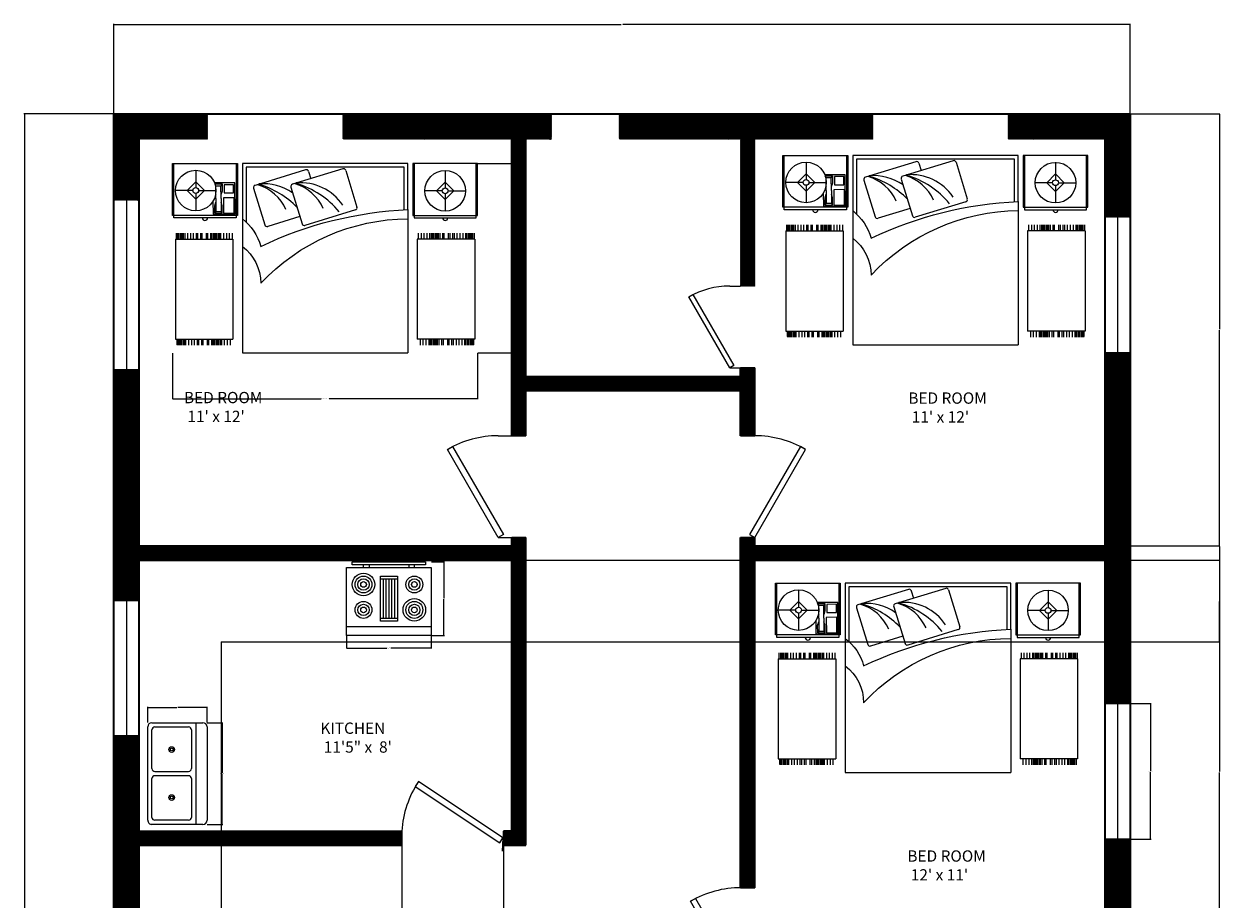
# Model space of a CAD drawing. Units: inches. Extents: x -19 to 404, y -21 to 673.
# Tile 3 of 3: x -19 to 404, y 363 to 673. Entities that reach past the tile are written whole.
import ezdxf

# ---------------------------------------------------------------- set-up
doc = ezdxf.new("R2010")
doc.units = ezdxf.units.IN
doc.header["$MEASUREMENT"] = 0
for name, color, linetype, lineweight in [('A-ANNO-DIMS', 2, 'Continuous', 18), ('A-AREA-IDEN', 7, 'Continuous', 18), ('A-WALL', 7, 'Continuous', 35), ('bedroom', 120, 'Continuous', 18), ('doors', 40, 'Continuous', 18), ('kitchen', 181, 'Continuous', 18), ('window', 30, 'Continuous', 18)]:
    doc.layers.add(name, color=color, linetype=linetype, lineweight=lineweight)
doc.layers.add('A-WALL-PATT', color=244, linetype='Continuous', lineweight=13, true_color=0x991b1e)
doc.styles.get("Standard").update_dxf_attribs({"font": 'arial.ttf'})
doc.dimstyles.get("Standard").update_dxf_attribs({"dimtxt": 0.18, "dimasz": 0.18, "dimexe": 0.18, "dimexo": 0.0625, "dimgap": 0.09, "dimtad": 0, "dimtih": 1, "dimtoh": 1, "dimdec": 4, "dimzin": 0, "dimdsep": 46, "dimtxsty": 'Standard', "dimcen": 0.09, "dimadec": 0, "dimazin": 0, "dimtfac": 1, "dimtdec": 4, "dimtofl": 0, "dimtmove": 0, "dimatfit": 3, "dimfxl": 1, "dimtolj": 1, "dimtzin": 0, "dimarcsym": 0})
pattern_1 = [(45, (-13642.13922, -42713.83606), (-0.08838834765, 0.08838834765), [])]

# ---------------------------------------------------------------- blocks, each defined once
blk = doc.blocks.new('*U5')
for p, q in [((0, 0), (0, -100)), ((750, 0), (750, -100))]:
    blk.add_line(p, q)
blk.add_lwpolyline([(0, 0), (649.5, 375), (671.4, 337.1), (21.9, -37.9)], close=True)
blk.add_arc((0, 0), 750, 0, 30)
blk = doc.blocks.new('*U6')
for p, q in [((0, 0), (0, 100)), ((750, 0), (750, 100))]:
    blk.add_line(p, q)
blk.add_lwpolyline([(0, 0), (649.5, -375), (671.4, -337.1), (21.9, 37.9)], close=True)
blk.add_arc((0, 0), 750, 330, 0)
blk = doc.blocks.new('3')
for p, q in [((185.866, 224.677), (185.866, 225.236)), ((185.866, 225.236), (186.566, 225.236)), ((185.88, 224.649), (185.88, 225.236)), ((186.552, 225.236), (186.552, 224.649)), ((186.566, 225.236), (186.566, 224.677)), ((186.62, 225.236), (186.62, 224.64)), ((188.409, 225.236), (186.62, 225.236)), ((188.409, 224.739), (188.409, 225.236)), ((188.463, 225.236), (188.463, 224.677)), ((189.162, 225.236), (188.463, 225.236)), ((188.477, 225.236), (188.477, 224.649)), ((189.148, 224.649), (189.148, 225.236)), ((189.162, 224.677), (189.162, 225.236)), ((186.116, 225.164), (186.116, 224.976)), ((187.303, 225.168), (186.758, 225.001)), ((187.706, 225.179), (187.161, 225.012)), ((187.334, 225.152), (187.359, 225.073)), ((187.737, 225.163), (187.858, 224.766)), ((188.812, 225.162), (188.812, 224.974)), ((186.084, 224.945), (185.896, 224.945)), ((186.022, 224.945), (186.116, 225.039)), ((186.116, 224.851), (186.022, 224.945)), ((186.116, 225.039), (186.21, 224.945)), ((186.21, 224.945), (186.116, 224.851)), ((186.147, 224.945), (186.335, 224.945)), ((186.54, 225.027), (186.319, 225.027)), ((186.321, 225.017), (186.401, 225.017)), ((186.333, 224.997), (186.321, 225.017)), ((186.334, 224.858), (186.333, 224.997)), ((186.333, 224.997), (186.389, 224.997)), ((186.401, 225.017), (186.389, 224.997)), ((186.39, 224.858), (186.389, 224.997)), ((186.401, 224.938), (186.389, 224.898)), ((186.401, 225.017), (186.401, 224.938)), ((186.541, 224.69), (186.54, 225.027)), ((186.742, 224.97), (186.863, 224.573)), ((187.144, 224.981), (187.266, 224.584)), ((188.781, 224.942), (188.593, 224.942)), ((188.812, 225.036), (188.718, 224.942)), ((188.718, 224.942), (188.812, 224.848)), ((188.907, 224.942), (188.812, 225.036)), ((188.812, 224.848), (188.907, 224.942)), ((188.844, 224.942), (189.032, 224.942)), ((186.116, 224.914), (186.116, 224.726)), ((186.302, 224.83), (186.303, 224.689)), ((186.322, 224.779), (186.334, 224.818)), ((186.331, 224.905), (186.334, 224.898)), ((186.334, 224.858), (186.334, 224.719)), ((186.39, 224.858), (186.39, 224.719)), ((186.402, 224.779), (186.39, 224.819)), ((188.812, 224.911), (188.812, 224.723)), ((186.566, 224.677), (185.866, 224.677)), ((186.303, 224.689), (186.541, 224.69)), ((186.323, 224.699), (186.322, 224.779)), ((186.334, 224.719), (186.323, 224.699)), ((186.323, 224.699), (186.402, 224.7)), ((186.334, 224.719), (186.39, 224.719)), ((186.402, 224.7), (186.39, 224.719)), ((186.402, 224.7), (186.402, 224.779)), ((187.842, 224.735), (187.297, 224.568)), ((188.409, 224.739), (188.409, 223.191)), ((188.463, 224.677), (189.162, 224.677)), ((186.552, 224.649), (185.88, 224.649)), ((186.62, 224.64), (186.62, 223.191)), ((187.242, 224.663), (186.894, 224.557)), ((188.477, 224.649), (189.148, 224.649)), ((185.897, 224.42, -0.909), (185.897, 223.338, -0.909)), ((185.897, 224.42, -0.909), (186.517, 224.42, -0.909)), ((185.904, 224.485, -0.909), (185.904, 224.42, -0.909)), ((185.92, 224.485, -0.909), (185.92, 224.42, -0.909)), ((185.92, 224.485, -0.909), (185.92, 224.42, -0.909)), ((185.935, 224.485, -0.909), (185.935, 224.42, -0.909)), ((185.951, 224.485, -0.909), (185.951, 224.42, -0.909)), ((185.966, 224.485, -0.909), (185.966, 224.42, -0.909)), ((185.982, 224.485, -0.909), (185.982, 224.42, -0.909)), ((185.997, 224.485, -0.909), (185.997, 224.42, -0.909)), ((186.028, 224.485, -0.909), (186.028, 224.42, -0.909)), ((186.059, 224.485, -0.909), (186.059, 224.42, -0.909)), ((186.09, 224.485, -0.909), (186.09, 224.42, -0.909)), ((186.09, 224.485, -0.909), (186.09, 224.42, -0.909)), ((186.121, 224.485, -0.909), (186.121, 224.42, -0.909)), ((186.137, 224.485, -0.909), (186.137, 224.42, -0.909)), ((186.168, 224.485, -0.909), (186.168, 224.42, -0.909)), ((186.183, 224.485, -0.909), (186.183, 224.42, -0.909)), ((186.23, 224.485, -0.909), (186.23, 224.42, -0.909)), ((186.245, 224.485, -0.909), (186.245, 224.42, -0.909)), ((186.276, 224.485, -0.909), (186.276, 224.42, -0.909)), ((186.292, 224.485, -0.909), (186.292, 224.42, -0.909)), ((186.307, 224.485, -0.909), (186.307, 224.42, -0.909)), ((186.323, 224.485, -0.909), (186.323, 224.42, -0.909)), ((186.338, 224.485, -0.909), (186.338, 224.42, -0.909)), ((186.354, 224.485, -0.909), (186.354, 224.42, -0.909)), ((186.369, 224.485, -0.909), (186.369, 224.42, -0.909)), ((186.385, 224.485, -0.909), (186.385, 224.42, -0.909)), ((186.416, 224.485, -0.909), (186.416, 224.42, -0.909)), ((186.447, 224.485, -0.909), (186.447, 224.42, -0.909)), ((186.478, 224.485, -0.909), (186.478, 224.42, -0.909)), ((186.509, 224.485, -0.909), (186.509, 224.42, -0.909)), ((186.517, 224.42, -0.909), (186.517, 223.338, -0.909)), ((189.131, 224.42, -0.909), (188.511, 224.42, -0.909)), ((188.511, 224.42, -0.909), (188.511, 223.338, -0.909)), ((188.52, 224.485, -0.909), (188.52, 224.42, -0.909)), ((188.551, 224.485, -0.909), (188.551, 224.42, -0.909)), ((188.582, 224.485, -0.909), (188.582, 224.42, -0.909)), ((188.613, 224.485, -0.909), (188.613, 224.42, -0.909)), ((188.644, 224.485, -0.909), (188.644, 224.42, -0.909)), ((188.66, 224.485, -0.909), (188.66, 224.42, -0.909)), ((188.675, 224.485, -0.909), (188.675, 224.42, -0.909)), ((188.691, 224.485, -0.909), (188.691, 224.42, -0.909)), ((188.706, 224.485, -0.909), (188.706, 224.42, -0.909)), ((188.722, 224.485, -0.909), (188.722, 224.42, -0.909)), ((188.737, 224.485, -0.909), (188.737, 224.42, -0.909)), ((188.753, 224.485, -0.909), (188.753, 224.42, -0.909)), ((188.784, 224.485, -0.909), (188.784, 224.42, -0.909)), ((188.799, 224.485, -0.909), (188.799, 224.42, -0.909)), ((188.846, 224.485, -0.909), (188.846, 224.42, -0.909)), ((188.861, 224.485, -0.909), (188.861, 224.42, -0.909)), ((188.892, 224.485, -0.909), (188.892, 224.42, -0.909)), ((188.908, 224.485, -0.909), (188.908, 224.42, -0.909)), ((188.939, 224.485, -0.909), (188.939, 224.42, -0.909)), ((188.939, 224.485, -0.909), (188.939, 224.42, -0.909)), ((188.97, 224.485, -0.909), (188.97, 224.42, -0.909)), ((189.001, 224.485, -0.909), (189.001, 224.42, -0.909)), ((189.032, 224.485, -0.909), (189.032, 224.42, -0.909)), ((189.047, 224.485, -0.909), (189.047, 224.42, -0.909)), ((189.063, 224.485, -0.909), (189.063, 224.42, -0.909)), ((189.078, 224.485, -0.909), (189.078, 224.42, -0.909)), ((189.094, 224.485, -0.909), (189.094, 224.42, -0.909)), ((189.109, 224.485, -0.909), (189.109, 224.42, -0.909)), ((189.109, 224.485, -0.909), (189.109, 224.42, -0.909)), ((189.125, 224.485, -0.909), (189.125, 224.42, -0.909)), ((189.131, 224.42, -0.909), (189.131, 223.338, -0.909)), ((185.897, 223.338, -0.909), (186.517, 223.338, -0.909)), ((185.911, 223.338, -0.909), (185.911, 223.279, -0.909)), ((185.911, 223.338, -0.909), (185.911, 223.279, -0.909)), ((185.911, 223.338, -0.909), (185.911, 223.279, -0.909)), ((185.914, 223.338, -0.909), (185.914, 223.273, -0.909)), ((185.929, 223.338, -0.909), (185.929, 223.273, -0.909)), ((185.929, 223.338, -0.909), (185.929, 223.273, -0.909)), ((185.945, 223.338, -0.909), (185.945, 223.273, -0.909)), ((185.96, 223.338, -0.909), (185.96, 223.273, -0.909)), ((185.976, 223.338, -0.909), (185.976, 223.273, -0.909)), ((185.991, 223.338, -0.909), (185.991, 223.273, -0.909)), ((186.007, 223.338, -0.909), (186.007, 223.273, -0.909)), ((186.038, 223.338, -0.909), (186.038, 223.273, -0.909)), ((186.069, 223.338, -0.909), (186.069, 223.273, -0.909)), ((186.1, 223.338, -0.909), (186.1, 223.273, -0.909)), ((186.1, 223.338, -0.909), (186.1, 223.273, -0.909)), ((186.131, 223.338, -0.909), (186.131, 223.273, -0.909)), ((186.146, 223.338, -0.909), (186.146, 223.273, -0.909)), ((186.177, 223.338, -0.909), (186.177, 223.273, -0.909)), ((186.193, 223.338, -0.909), (186.193, 223.273, -0.909)), ((186.239, 223.338, -0.909), (186.239, 223.273, -0.909)), ((186.255, 223.338, -0.909), (186.255, 223.273, -0.909)), ((186.286, 223.338, -0.909), (186.286, 223.273, -0.909)), ((186.301, 223.338, -0.909), (186.301, 223.273, -0.909)), ((186.317, 223.338, -0.909), (186.317, 223.273, -0.909)), ((186.332, 223.338, -0.909), (186.332, 223.273, -0.909)), ((186.348, 223.338, -0.909), (186.348, 223.273, -0.909)), ((186.363, 223.338, -0.909), (186.363, 223.273, -0.909)), ((186.379, 223.338, -0.909), (186.379, 223.273, -0.909)), ((186.394, 223.338, -0.909), (186.394, 223.273, -0.909)), ((186.425, 223.338, -0.909), (186.425, 223.273, -0.909)), ((186.456, 223.338, -0.909), (186.456, 223.273, -0.909)), ((186.487, 223.338, -0.909), (186.487, 223.273, -0.909)), ((189.131, 223.338, -0.909), (188.511, 223.338, -0.909)), ((188.541, 223.338, -0.909), (188.541, 223.273, -0.909)), ((188.572, 223.338, -0.909), (188.572, 223.273, -0.909)), ((188.603, 223.338, -0.909), (188.603, 223.273, -0.909)), ((188.634, 223.338, -0.909), (188.634, 223.273, -0.909)), ((188.65, 223.338, -0.909), (188.65, 223.273, -0.909)), ((188.665, 223.338, -0.909), (188.665, 223.273, -0.909)), ((188.681, 223.338, -0.909), (188.681, 223.273, -0.909)), ((188.696, 223.338, -0.909), (188.696, 223.273, -0.909)), ((188.712, 223.338, -0.909), (188.712, 223.273, -0.909)), ((188.727, 223.338, -0.909), (188.727, 223.273, -0.909)), ((188.743, 223.338, -0.909), (188.743, 223.273, -0.909)), ((188.774, 223.338, -0.909), (188.774, 223.273, -0.909)), ((188.789, 223.338, -0.909), (188.789, 223.273, -0.909)), ((188.836, 223.338, -0.909), (188.836, 223.273, -0.909)), ((188.851, 223.338, -0.909), (188.851, 223.273, -0.909)), ((188.882, 223.338, -0.909), (188.882, 223.273, -0.909)), ((188.898, 223.338, -0.909), (188.898, 223.273, -0.909)), ((188.929, 223.338, -0.909), (188.929, 223.273, -0.909)), ((188.929, 223.338, -0.909), (188.929, 223.273, -0.909)), ((188.96, 223.338, -0.909), (188.96, 223.273, -0.909)), ((188.991, 223.338, -0.909), (188.991, 223.273, -0.909)), ((189.022, 223.338, -0.909), (189.022, 223.273, -0.909)), ((189.037, 223.338, -0.909), (189.037, 223.273, -0.909)), ((189.053, 223.338, -0.909), (189.053, 223.273, -0.909)), ((189.068, 223.338, -0.909), (189.068, 223.273, -0.909)), ((189.084, 223.338, -0.909), (189.084, 223.273, -0.909)), ((189.099, 223.338, -0.909), (189.099, 223.273, -0.909)), ((189.099, 223.338, -0.909), (189.099, 223.273, -0.909)), ((189.115, 223.338, -0.909), (189.115, 223.273, -0.909)), ((189.117, 223.338, -0.909), (189.117, 223.279, -0.909)), ((189.117, 223.338, -0.909), (189.117, 223.279, -0.909)), ((189.117, 223.338, -0.909), (189.117, 223.279, -0.909)), ((186.62, 223.191), (188.409, 223.191))]:
    blk.add_line(p, q)
blk.add_lwpolyline([(188.369, 224.737), (188.369, 225.197), (186.66, 225.197), (186.66, 224.606)])
for points in [[(186.422, 225.007), (186.422, 224.92), (186.525, 224.92), (186.525, 225.008)], [(186.415, 224.866), (186.416, 224.7), (186.531, 224.7), (186.53, 224.867)]]:
    blk.add_lwpolyline(points, close=True)
for points in [[(186.62, 224.64, -0.162278), (186.819, 224.342, -0.100664), (188.409, 224.739, -0.100664)], [(186.62, 224.342, -0.236068), (186.819, 223.944, -0.205258), (188.409, 224.64, -0.205258)]]:
    blk.add_lwpolyline(points, format="xyb")
for centre, radius in [((186.116, 224.945), 0.219), ((188.812, 224.942), 0.219), ((186.116, 224.945), 0.0313), ((188.812, 224.942), 0.0313)]:
    blk.add_circle(centre, radius)
for centre, radius, start, end in [((187.311, 225.145), 0.0248, 17.0142, 107.0142), ((187.713, 225.156), 0.0248, 17.0142, 107.0142), ((186.765, 224.978), 0.0248, 107.0142, 197.0142), ((186.647, 224.541), 0.487, 24.2209, 73.0691), ((186.848, 224.471), 0.547, 54.6851, 95.1605), ((186.536, 224.105), 0.943, 44.2727, 73.7189), ((187.168, 224.989), 0.0248, 107.0142, 197.0142), ((187.05, 224.552), 0.487, 24.2209, 73.0691), ((187.25, 224.482), 0.547, 33.7801, 95.1605), ((186.938, 224.116), 0.943, 39.4023, 73.7189), ((187.835, 224.758), 0.0248, 287.0142, 17.0142), ((186.216, 224.649), 0.028, 180, 0), ((186.887, 224.581), 0.0248, 197.0142, 287.0142), ((187.289, 224.592), 0.0248, 197.0142, 287.0142), ((188.812, 224.649), 0.028, 180, 0)]:
    blk.add_arc(centre, radius, start, end)
blk = doc.blocks.new('Sink-double - 36 in top')
for p, q in [((-18, -4), (18, -4)), ((-0.75, -18.5), (-0.75, -6.5)), ((0.75, -6.5), (0.75, -18.5))]:
    blk.add_line(p, q)
for points in [[(-16.5, 0), (16.5, 0)], [(-18, -19.5), (-18, -1.5)], [(18, -1.5), (18, -19.5)], [(-16.5, -18.5), (-16.5, -6.5)], [(-15.5, -5.5), (-1.75, -5.5)], [(1.75, -5.5), (15.5, -5.5)], [(16.5, -6.5), (16.5, -18.5)], [(16.5, -21), (-16.5, -21)], [(-1.75, -19.5), (-15.5, -19.5)], [(15.5, -19.5), (1.75, -19.5)]]:
    blk.add_lwpolyline(points)
for centre, radius in [((-8.5, -12.5), 1), ((-8.5, -12.5), 0.5), ((8.5, -12.5), 1), ((8.5, -12.5), 0.5)]:
    blk.add_circle(centre, radius)
for centre, radius, start, end in [((-16.5, -1.5), 1.5, 90, 180), ((16.5, -1.5), 1.5, 0, 90), ((-15.5, -6.5), 1, 90, 180), ((-1.75, -6.5), 1, 0, 90), ((1.75, -6.5), 1, 90, 180), ((15.5, -6.5), 1, 0, 90), ((-16.5, -19.5), 1.5, 180, 270), ((-15.5, -18.5), 1, 180, 270), ((-1.75, -18.5), 1, 270, 0), ((1.75, -18.5), 1, 180, 270), ((15.5, -18.5), 1, 270, 0), ((16.5, -19.5), 1.5, 270, 0)]:
    blk.add_arc(centre, radius, start, end)
blk = doc.blocks.new('Range-Oven - 30 in top')
for p, q in [((0, -3), (30, -3)), ((12, -6), (18, -6)), ((13, -20), (13, -6)), ((14, -6), (14, -20)), ((15, -20), (15, -6)), ((16, -6), (16, -20)), ((17, -20), (17, -6)), ((18, -20), (12, -20)), ((6, -24), (6, -25)), ((8, -25), (8, -24)), ((22, -25), (22, -24)), ((24, -24), (24, -25))]:
    blk.add_line(p, q)
for points in [[(0, -24), (0, 0), (30, 0), (30, -24)], [(12, -21), (12, -5), (18, -5), (18, -21)], [(2, -26), (2, -25), (28, -25), (28, -26)]]:
    blk.add_lwpolyline(points, close=True)
for centre, radius in [((6, -9), 4), ((6, -9), 3), ((6, -9), 2), ((6, -9), 1), ((24, -9), 3), ((24, -9), 2), ((24, -9), 1), ((6, -18), 3), ((6, -18), 2), ((24, -18), 4), ((24, -18), 3), ((24, -18), 2), ((6, -18), 1), ((24, -18), 1)]:
    blk.add_circle(centre, radius)
blk = doc.blocks.new('WIN-48IN')
for p, q in [((0, 48), (9, 48)), ((0, 0), (0, 48)), ((0, 48), (4.5, 48)), ((4.5, 48), (4.5, 0)), ((9, 48), (9, 0)), ((9, 0), (0, 0))]:
    blk.add_line(p, q)
blk = doc.blocks.new('*D11')
at = {"layer": 'A-ANNO-DIMS', "color": 0, "lineweight": -2, "transparency": 16777216}
for p, q in [((33.51, 556.07), (33.51, 539.75)), ((141.51, 556.07), (141.51, 539.75)), ((33.69, 539.93), (86.12, 539.93)), ((141.33, 539.93), (88.89, 539.93))]:
    blk.add_line(p, q, dxfattribs=at)
at = {"layer": 'A-ANNO-DIMS', "color": 0, "transparency": 16777216}
for points in [[(33.69, 539.96), (33.69, 539.9), (33.51, 539.93)], [(141.33, 539.96), (141.33, 539.9), (141.51, 539.93)]]:
    blk.add_solid(points, dxfattribs=at)
at = {"layer": 'Defpoints', "color": 0, "transparency": 16777216}
for p in [(33.51, 556.13), (141.51, 556.13), (141.51, 539.93)]:
    blk.add_point(p, dxfattribs=at)
at = {"layer": 'A-ANNO-DIMS', "color": 0, "transparency": 16777216, "insert": (87.51, 539.93), "char_height": 0.18, "attachment_point": 5}
blk.add_mtext('\\A1;BED GROUP 108 TYP.', dxfattribs=at)
blk = doc.blocks.new('*D12')
at = {"layer": 'A-ANNO-DIMS', "color": 0, "lineweight": -2, "transparency": 16777216}
for p, q in [((141.57, 623.16), (157.89, 623.16)), ((157.71, 622.98), (157.71, 589.83)), ((157.71, 556.31), (157.71, 589.46)), ((141.57, 556.13), (157.89, 556.13))]:
    blk.add_line(p, q, dxfattribs=at)
at = {"layer": 'A-ANNO-DIMS', "color": 0, "transparency": 16777216}
for points in [[(157.68, 622.98), (157.74, 622.98), (157.71, 623.16)], [(157.68, 556.31), (157.74, 556.31), (157.71, 556.13)]]:
    blk.add_solid(points, dxfattribs=at)
at = {"layer": 'Defpoints', "color": 0, "transparency": 16777216}
for p in [(141.51, 623.16), (157.71, 623.16), (141.51, 556.13)]:
    blk.add_point(p, dxfattribs=at)
at = {"layer": 'A-ANNO-DIMS', "color": 0, "transparency": 16777216, "insert": (157.71, 589.64), "char_height": 0.18, "attachment_point": 5}
blk.add_mtext('\\A1;67 TYP.', dxfattribs=at)
blk = doc.blocks.new('*D13')
at = {"layer": 'A-ANNO-DIMS', "color": 0, "lineweight": -2, "transparency": 16777216}
for p, q in [((372.71, 431.98), (380.03, 431.98)), ((379.85, 431.8), (379.85, 408.17)), ((379.85, 384.16), (379.85, 407.8)), ((372.71, 383.98), (380.03, 383.98))]:
    blk.add_line(p, q, dxfattribs=at)
at = {"layer": 'A-ANNO-DIMS', "color": 0, "transparency": 16777216}
for points in [[(379.82, 431.8), (379.88, 431.8), (379.85, 431.98)], [(379.82, 384.16), (379.88, 384.16), (379.85, 383.98)]]:
    blk.add_solid(points, dxfattribs=at)
at = {"layer": 'Defpoints', "color": 0, "transparency": 16777216}
for p in [(372.65, 431.98), (379.85, 431.98), (372.65, 383.98)]:
    blk.add_point(p, dxfattribs=at)
at = {"layer": 'A-ANNO-DIMS', "color": 0, "transparency": 16777216, "insert": (379.85, 407.98), "char_height": 0.18, "attachment_point": 5}
blk.add_mtext('\\A1;WINDOW 48 TYP.', dxfattribs=at)
blk = doc.blocks.new('*D14')
at = {"layer": 'A-ANNO-DIMS', "color": 0, "lineweight": -2, "transparency": 16777216}
for p, q in [((363.65, 383.92), (363.65, 376.6)), ((372.65, 383.92), (372.65, 376.6)), ((363.83, 376.78), (367.69, 376.78)), ((372.47, 376.78), (368.61, 376.78))]:
    blk.add_line(p, q, dxfattribs=at)
at = {"layer": 'A-ANNO-DIMS', "color": 0, "transparency": 16777216}
for points in [[(363.83, 376.81), (363.83, 376.75), (363.65, 376.78)], [(372.47, 376.81), (372.47, 376.75), (372.65, 376.78)]]:
    blk.add_solid(points, dxfattribs=at)
at = {"layer": 'Defpoints', "color": 0, "transparency": 16777216}
for p in [(363.65, 383.98), (372.65, 383.98), (372.65, 376.78)]:
    blk.add_point(p, dxfattribs=at)
at = {"layer": 'A-ANNO-DIMS', "color": 0, "transparency": 16777216, "insert": (368.15, 376.78), "char_height": 0.18, "attachment_point": 5}
blk.add_mtext('\\A1;9 TYP.', dxfattribs=at)
blk = doc.blocks.new('*D21')
at = {"layer": 'A-ANNO-DIMS', "color": 0, "lineweight": -2, "transparency": 16777216}
for p, q in [((45.75, 425.23), (51.27, 425.23)), ((51.09, 425.05), (51.09, 407.41)), ((51.09, 389.41), (51.09, 407.04)), ((45.75, 389.23), (51.27, 389.23))]:
    blk.add_line(p, q, dxfattribs=at)
at = {"layer": 'A-ANNO-DIMS', "color": 0, "transparency": 16777216}
for points in [[(51.06, 425.05), (51.12, 425.05), (51.09, 425.23)], [(51.06, 389.41), (51.12, 389.41), (51.09, 389.23)]]:
    blk.add_solid(points, dxfattribs=at)
at = {"layer": 'Defpoints', "color": 0, "transparency": 16777216}
for p in [(45.69, 425.23), (45.69, 389.23), (51.09, 389.23)]:
    blk.add_point(p, dxfattribs=at)
at = {"layer": 'A-ANNO-DIMS', "color": 0, "transparency": 16777216, "insert": (51.09, 407.23), "char_height": 0.18, "attachment_point": 5}
blk.add_mtext('\\A1;DOUBLE SINK 36', dxfattribs=at)
blk = doc.blocks.new('*D22')
at = {"layer": 'A-ANNO-DIMS', "color": 0, "lineweight": -2, "transparency": 16777216}
for p, q in [((24.69, 425.29), (24.69, 430.81)), ((24.87, 430.63), (34.99, 430.63)), ((45.51, 430.63), (35.39, 430.63)), ((45.69, 425.29), (45.69, 430.81))]:
    blk.add_line(p, q, dxfattribs=at)
at = {"layer": 'A-ANNO-DIMS', "color": 0, "transparency": 16777216}
for points in [[(24.87, 430.66), (24.87, 430.6), (24.69, 430.63)], [(45.51, 430.66), (45.51, 430.6), (45.69, 430.63)]]:
    blk.add_solid(points, dxfattribs=at)
at = {"layer": 'Defpoints', "color": 0, "transparency": 16777216}
for p in [(45.69, 430.63), (24.69, 425.23), (45.69, 425.23)]:
    blk.add_point(p, dxfattribs=at)
at = {"layer": 'A-ANNO-DIMS', "color": 0, "transparency": 16777216, "insert": (35.19, 430.63), "char_height": 0.18, "attachment_point": 5}
blk.add_mtext('\\A1;21', dxfattribs=at)
blk = doc.blocks.new('*D23')
at = {"layer": 'A-ANNO-DIMS', "color": 0, "lineweight": -2, "transparency": 16777216}
for p, q in [((95.11, 456.1), (95.11, 451.48)), ((125.11, 456.1), (125.11, 451.48)), ((95.29, 451.66), (109.42, 451.66)), ((124.93, 451.66), (110.81, 451.66))]:
    blk.add_line(p, q, dxfattribs=at)
at = {"layer": 'A-ANNO-DIMS', "color": 0, "transparency": 16777216}
for points in [[(95.29, 451.69), (95.29, 451.63), (95.11, 451.66)], [(124.93, 451.69), (124.93, 451.63), (125.11, 451.66)]]:
    blk.add_solid(points, dxfattribs=at)
at = {"layer": 'Defpoints', "color": 0, "transparency": 16777216}
for p in [(95.11, 456.16), (125.11, 456.16), (95.11, 451.66)]:
    blk.add_point(p, dxfattribs=at)
at = {"layer": 'A-ANNO-DIMS', "color": 0, "transparency": 16777216, "insert": (110.11, 451.66), "char_height": 0.18, "attachment_point": 5}
blk.add_mtext('\\A1;RANGE 30', dxfattribs=at)
blk = doc.blocks.new('*D24')
at = {"layer": 'A-ANNO-DIMS', "color": 0, "lineweight": -2, "transparency": 16777216}
for p, q in [((125.17, 482.16), (129.79, 482.16)), ((129.61, 481.98), (129.61, 469.35)), ((129.61, 456.34), (129.61, 468.98)), ((125.17, 456.16), (129.79, 456.16))]:
    blk.add_line(p, q, dxfattribs=at)
at = {"layer": 'A-ANNO-DIMS', "color": 0, "transparency": 16777216}
for points in [[(129.58, 481.98), (129.64, 481.98), (129.61, 482.16)], [(129.58, 456.34), (129.64, 456.34), (129.61, 456.16)]]:
    blk.add_solid(points, dxfattribs=at)
at = {"layer": 'Defpoints', "color": 0, "transparency": 16777216}
for p in [(125.11, 482.16), (125.11, 456.16), (129.61, 456.16)]:
    blk.add_point(p, dxfattribs=at)
at = {"layer": 'A-ANNO-DIMS', "color": 0, "transparency": 16777216, "insert": (129.61, 469.16), "char_height": 0.18, "attachment_point": 5}
blk.add_mtext('\\A1;26', dxfattribs=at)
blk = doc.blocks.new('*D25')
at = {"layer": 'A-ANNO-DIMS', "color": 0, "lineweight": -2, "transparency": 16777216}
for p, q in [((12.65, 640.88), (12.65, 672.6)), ((12.83, 672.42), (192.36, 672.42)), ((372.47, 672.42), (192.94, 672.42)), ((372.65, 640.88), (372.65, 672.6))]:
    blk.add_line(p, q, dxfattribs=at)
at = {"layer": 'A-ANNO-DIMS', "color": 0, "transparency": 16777216}
for points in [[(12.83, 672.45), (12.83, 672.39), (12.65, 672.42)], [(372.47, 672.45), (372.47, 672.39), (372.65, 672.42)]]:
    blk.add_solid(points, dxfattribs=at)
at = {"layer": 'Defpoints', "color": 0, "transparency": 16777216}
for p in [(372.65, 672.42), (12.65, 640.82), (372.65, 640.82)]:
    blk.add_point(p, dxfattribs=at)
at = {"layer": 'A-ANNO-DIMS', "color": 0, "transparency": 16777216, "insert": (192.65, 672.42), "char_height": 0.18, "attachment_point": 5}
blk.add_mtext('\\A1;360', dxfattribs=at)
blk = doc.blocks.new('*D26')
at = {"layer": 'A-ANNO-DIMS', "color": 0, "lineweight": -2, "transparency": 16777216}
for p, q in [((12.59, 640.82), (-19.13, 640.82)), ((-18.95, 640.64), (-18.95, 326)), ((-18.95, 11), (-18.95, 325.64)), ((114.59, 10.82), (-19.13, 10.82))]:
    blk.add_line(p, q, dxfattribs=at)
at = {"layer": 'A-ANNO-DIMS', "color": 0, "transparency": 16777216}
for points in [[(-18.98, 640.64), (-18.92, 640.64), (-18.95, 640.82)], [(-18.98, 11), (-18.92, 11), (-18.95, 10.82)]]:
    blk.add_solid(points, dxfattribs=at)
at = {"layer": 'Defpoints', "color": 0, "transparency": 16777216}
for p in [(12.65, 640.82), (-18.95, 10.82), (114.65, 10.82)]:
    blk.add_point(p, dxfattribs=at)
at = {"layer": 'A-ANNO-DIMS', "color": 0, "transparency": 16777216, "insert": (-18.95, 325.82), "char_height": 0.18, "attachment_point": 5}
blk.add_mtext('\\A1;630', dxfattribs=at)
blk = doc.blocks.new('*D32')
at = {"layer": 'A-ANNO-DIMS', "color": 0, "lineweight": -2, "transparency": 16777216}
for p, q in [((372.71, 640.82), (404.42, 640.82)), ((404.24, 640.64), (404.24, 564.5)), ((404.24, 488), (404.24, 564.14)), ((363.71, 487.82), (404.42, 487.82))]:
    blk.add_line(p, q, dxfattribs=at)
at = {"layer": 'A-ANNO-DIMS', "color": 0, "transparency": 16777216}
for points in [[(404.21, 640.64), (404.27, 640.64), (404.24, 640.82)], [(404.21, 488), (404.27, 488), (404.24, 487.82)]]:
    blk.add_solid(points, dxfattribs=at)
at = {"layer": 'Defpoints', "color": 0, "transparency": 16777216}
for p in [(372.65, 640.82), (404.24, 640.82), (363.65, 487.82)]:
    blk.add_point(p, dxfattribs=at)
at = {"layer": 'A-ANNO-DIMS', "color": 0, "transparency": 16777216, "insert": (404.24, 564.32), "char_height": 0.18, "attachment_point": 5}
blk.add_mtext('\\A1;153', dxfattribs=at)
blk = doc.blocks.new('*D33')
at = {"layer": 'A-ANNO-DIMS', "color": 0, "lineweight": -2, "transparency": 16777216}
for p, q in [((363.71, 487.82), (404.42, 487.82)), ((404.24, 487.64), (404.24, 408)), ((404.24, 328), (404.24, 407.64)), ((363.71, 327.82), (404.42, 327.82))]:
    blk.add_line(p, q, dxfattribs=at)
at = {"layer": 'A-ANNO-DIMS', "color": 0, "transparency": 16777216}
for points in [[(404.21, 487.64), (404.27, 487.64), (404.24, 487.82)], [(404.21, 328), (404.27, 328), (404.24, 327.82)]]:
    blk.add_solid(points, dxfattribs=at)
at = {"layer": 'Defpoints', "color": 0, "transparency": 16777216}
for p in [(363.65, 487.82), (404.24, 487.82), (363.65, 327.82)]:
    blk.add_point(p, dxfattribs=at)
at = {"layer": 'A-ANNO-DIMS', "color": 0, "transparency": 16777216, "insert": (404.24, 407.82), "char_height": 0.18, "attachment_point": 5}
blk.add_mtext('\\A1;160', dxfattribs=at)
blk = doc.blocks.new('*D38')
at = {"layer": 'A-ANNO-DIMS', "color": 0, "lineweight": -2, "transparency": 16777216}
for p, q in [((21.65, 386.76), (21.65, -20.95)), ((50.65, 386.76), (50.65, -20.95)), ((21.83, -20.77), (35.93, -20.77)), ((50.47, -20.77), (36.37, -20.77))]:
    blk.add_line(p, q, dxfattribs=at)
at = {"layer": 'A-ANNO-DIMS', "color": 0, "transparency": 16777216}
for points in [[(21.83, -20.74), (21.83, -20.8), (21.65, -20.77)], [(50.47, -20.74), (50.47, -20.8), (50.65, -20.77)]]:
    blk.add_solid(points, dxfattribs=at)
at = {"layer": 'Defpoints', "color": 0, "transparency": 16777216}
for p in [(21.65, 386.82), (50.65, 386.82), (50.65, -20.77)]:
    blk.add_point(p, dxfattribs=at)
at = {"layer": 'A-ANNO-DIMS', "color": 0, "transparency": 16777216, "insert": (36.15, -20.77), "char_height": 0.18, "attachment_point": 5}
blk.add_mtext('\\A1;29', dxfattribs=at)
blk = doc.blocks.new('*D39')
at = {"layer": 'A-ANNO-DIMS', "color": 0, "lineweight": -2, "transparency": 16777216}
for p, q in [((153.71, 482.82), (404.42, 482.82)), ((404.24, 482.64), (404.24, 468.5)), ((404.24, 454), (404.24, 468.14)), ((153.71, 453.82), (404.42, 453.82))]:
    blk.add_line(p, q, dxfattribs=at)
at = {"layer": 'A-ANNO-DIMS', "color": 0, "transparency": 16777216}
for points in [[(404.21, 482.64), (404.27, 482.64), (404.24, 482.82)], [(404.21, 454), (404.27, 454), (404.24, 453.82)]]:
    blk.add_solid(points, dxfattribs=at)
at = {"layer": 'Defpoints', "color": 0, "transparency": 16777216}
for p in [(153.65, 482.82), (404.24, 482.82), (153.65, 453.82)]:
    blk.add_point(p, dxfattribs=at)
at = {"layer": 'A-ANNO-DIMS', "color": 0, "transparency": 16777216, "insert": (404.24, 468.32), "char_height": 0.18, "attachment_point": 5}
blk.add_mtext('\\A1;29', dxfattribs=at)
blk = doc.blocks.new('*D40')
at = {"layer": 'A-ANNO-DIMS', "color": 0, "lineweight": -2, "transparency": 16777216}
for p, q in [((114.65, 381.76), (114.65, -20.95)), ((150.65, 381.76), (150.65, -20.95)), ((114.83, -20.77), (132.43, -20.77)), ((150.47, -20.77), (132.87, -20.77))]:
    blk.add_line(p, q, dxfattribs=at)
at = {"layer": 'A-ANNO-DIMS', "color": 0, "transparency": 16777216}
for points in [[(114.83, -20.74), (114.83, -20.8), (114.65, -20.77)], [(150.47, -20.74), (150.47, -20.8), (150.65, -20.77)]]:
    blk.add_solid(points, dxfattribs=at)
at = {"layer": 'Defpoints', "color": 0, "transparency": 16777216}
for p in [(114.65, 381.82), (150.65, 381.82), (150.65, -20.77)]:
    blk.add_point(p, dxfattribs=at)
at = {"layer": 'A-ANNO-DIMS', "color": 0, "transparency": 16777216, "insert": (132.65, -20.77), "char_height": 0.18, "attachment_point": 5}
blk.add_mtext('\\A1;36', dxfattribs=at)

msp = doc.modelspace()

# ---------------------------------------------------------------- hatches: boundary and pattern name
at = {"layer": 'A-WALL-PATT'}
h = msp.add_hatch(dxfattribs=at)
h.set_pattern_fill('ANSI31', color=256)
h.set_pattern_definition(pattern_1)
h.paths.add_polyline_path([(45.83, 640.82), (12.65, 640.82), (12.65, 610.17), (17.15, 610.17), (21.65, 610.17), (21.65, 631.82), (45.83, 631.82)])
h.paths.add_polyline_path([(21.65, 550.17), (12.65, 550.17), (12.65, 468.55), (17.15, 468.55), (21.65, 468.55), (21.65, 482.82), (153.65, 482.82), (153.65, 386.82), (150.65, 386.82), (150.65, 381.82), (158.65, 381.82), (158.65, 490.82), (153.65, 490.82), (153.65, 487.82), (21.65, 487.82)])
h.paths.add_polyline_path([(21.65, 420.55), (12.65, 420.55), (12.65, 351.11), (17.15, 351.11), (21.65, 351.11), (21.65, 381.82), (114.65, 381.82), (114.65, 386.82), (21.65, 386.82)])
h.paths.add_polyline_path([(21.65, 291.11), (12.65, 291.11), (12.65, 40.82), (35.81, 40.82), (35.81, 49.82), (21.65, 49.82)])
h.paths.add_polyline_path([(114.65, 185.82), (117.65, 185.82), (117.65, 190.82), (114.65, 190.82), (113.65, 190.82), (110.65, 190.82), (105.65, 190.82), (105.65, 49.82), (83.81, 49.82), (83.81, 40.82), (114.65, 40.82)])
h = msp.add_hatch(dxfattribs=at)
h.set_pattern_fill('ANSI31', color=256)
h.set_pattern_definition(pattern_1)
h.paths.add_polyline_path([(372.65, 640.82), (329.44, 640.82), (329.44, 631.82), (363.65, 631.82), (363.65, 604.18), (368.15, 604.18), (372.65, 604.18)])
h.paths.add_polyline_path([(281.44, 640.82), (191.65, 640.82), (191.65, 631.82), (234.65, 631.82), (234.65, 579.82), (239.65, 579.82), (239.65, 631.82), (281.44, 631.82)])
h.paths.add_polyline_path([(167.65, 640.82), (93.83, 640.82), (93.83, 631.82), (153.65, 631.82), (153.65, 526.82), (158.65, 526.82), (158.65, 542.82), (234.65, 542.82), (234.65, 526.82), (239.65, 526.82), (239.65, 550.82), (234.65, 550.82), (234.65, 547.82), (158.65, 547.82), (158.65, 631.82), (167.65, 631.82)])
h = msp.add_hatch(dxfattribs=at)
h.set_pattern_fill('ANSI31', color=256)
h.set_pattern_definition(pattern_1)
h.paths.add_polyline_path([(372.65, 556.18), (363.65, 556.18), (363.65, 487.82), (239.65, 487.82), (239.65, 490.82), (234.65, 490.82), (234.65, 487.82), (234.65, 366.82), (239.65, 366.82), (239.65, 482.82), (363.65, 482.82), (363.65, 431.98), (368.15, 431.98), (372.65, 431.98)])
h = msp.add_hatch(dxfattribs=at)
h.set_pattern_fill('ANSI31', color=256)
h.set_pattern_definition(pattern_1)
h.paths.add_polyline_path([(195.39, 49.82), (177.65, 49.82), (177.65, 40.82), (195.39, 40.82)])
h.paths.add_polyline_path([(276.02, 49.82), (239.65, 49.82), (239.65, 146.82), (234.65, 146.82), (234.65, 49.82), (219.39, 49.82), (219.39, 40.82), (276.02, 40.82)])
h.paths.add_polyline_path([(372.65, 87.37), (363.65, 87.37), (363.65, 49.82), (324.02, 49.82), (324.02, 40.82), (372.65, 40.82)])
h.paths.add_polyline_path([(372.65, 280.5), (363.65, 280.5), (363.65, 243.82), (271.65, 243.82), (271.65, 238.82), (274.65, 238.82), (274.65, 190.82), (161.65, 190.82), (161.65, 185.82), (234.65, 185.82), (234.65, 182.82), (239.65, 182.82), (239.65, 185.82), (282.65, 185.82), (282.65, 190.82), (279.65, 190.82), (279.65, 238.82), (363.65, 238.82), (363.65, 225.27), (368.15, 225.27), (372.65, 225.27)])
h.paths.add_polyline_path([(372.65, 201.27), (363.65, 201.27), (363.65, 190.82), (311.65, 190.82), (311.65, 185.82), (363.65, 185.82), (363.65, 135.37), (368.15, 135.37), (372.65, 135.37)])
h.paths.add_polyline_path([(372.65, 383.98), (363.65, 383.98), (363.65, 327.82), (239.65, 327.82), (239.65, 330.82), (234.65, 330.82), (234.65, 327.82), (234.65, 238.82), (242.65, 238.82), (242.65, 243.82), (239.65, 243.82), (239.65, 322.82), (363.65, 322.82), (363.65, 304.5), (368.15, 304.5), (372.65, 304.5)])

# ---------------------------------------------------------------- linework, layer by layer
at = {"layer": 'A-WALL'}
for p, q in [((21.65, 487.82), (21.65, 631.82)), ((153.65, 526.82), (153.65, 631.82)), ((153.65, 526.82), (153.65, 631.82)), ((158.65, 547.82), (158.65, 631.82)), ((158.65, 547.82), (158.65, 631.82)), ((363.65, 631.82), (363.65, 487.82)), ((234.65, 547.82), (234.65, 550.82)), ((234.65, 547.82), (234.65, 550.82)), ((234.65, 550.82), (239.65, 550.82)), ((239.65, 526.82), (239.65, 550.82)), ((158.65, 547.82), (234.65, 547.82)), ((158.65, 542.82), (234.65, 542.82)), ((158.65, 526.82), (158.65, 542.82)), ((158.65, 526.82), (158.65, 542.82)), ((234.65, 526.82), (234.65, 542.82)), ((158.65, 526.82), (153.65, 526.82)), ((239.65, 526.82), (234.65, 526.82)), ((21.65, 487.82), (153.65, 487.82)), ((153.65, 487.82), (153.65, 490.82)), ((153.65, 487.82), (153.65, 490.82)), ((153.65, 487.82), (153.65, 490.82)), ((153.65, 490.82), (158.65, 490.82)), ((158.65, 381.82), (158.65, 490.82)), ((158.65, 482.82), (158.65, 490.82)), ((234.65, 366.82), (234.65, 490.82)), ((234.65, 487.82), (234.65, 490.82)), ((234.65, 490.82), (239.65, 490.82)), ((239.65, 487.82), (239.65, 490.82)), ((239.65, 487.82), (363.65, 487.82)), ((21.65, 482.82), (153.65, 482.82)), ((21.65, 386.82), (21.65, 482.82)), ((153.65, 386.82), (153.65, 482.82)), ((239.65, 482.82), (363.65, 482.82)), ((239.65, 366.82), (239.65, 482.82)), ((363.65, 482.82), (363.65, 327.82)), ((21.65, 386.82), (114.65, 386.82)), ((114.65, 381.82), (114.65, 386.82)), ((150.65, 386.82), (153.65, 386.82)), ((153.65, 386.82), (150.65, 386.82)), ((150.65, 386.82), (150.65, 381.82)), ((21.65, 381.82), (114.65, 381.82)), ((21.65, 49.82), (21.65, 381.82)), ((150.65, 381.82), (158.65, 381.82)), ((239.65, 366.82), (234.65, 366.82))]:
    msp.add_line(p, q, dxfattribs=at)
msp.add_lwpolyline([(114.65, 40.82), (12.65, 40.82), (12.65, 640.82), (372.65, 640.82), (372.65, 40.82), (177.65, 40.82)], dxfattribs=at)
at = {"layer": 'kitchen'}
for p, q in [((21.65, 482.82), (21.65, 453.82)), ((21.65, 482.82), (50.65, 482.82)), ((50.65, 453.82), (153.65, 453.82)), ((50.65, 453.82), (50.65, 386.82))]:
    msp.add_line(p, q, dxfattribs=at)
at = {"layer": 'window'}
for p, q in [((12.65, 550.17), (12.65, 610.17)), ((17.15, 610.17), (17.15, 550.17)), ((21.65, 610.17), (21.65, 550.17)), ((363.65, 556.18), (363.65, 604.18)), ((368.15, 604.18), (368.15, 556.18)), ((372.65, 604.18), (372.65, 556.18)), ((372.65, 556.18), (363.65, 556.18)), ((21.65, 550.17), (12.65, 550.17))]:
    msp.add_line(p, q, dxfattribs=at)

# ---------------------------------------------------------------- block references
at = {"layer": 'bedroom', "xscale": 32.76894482774335, "yscale": 32.76894482774335, "zscale": 32.76894482774335}
for p in [(-6057.14, -6757.59), (-5841, -6754.71), (-5843.64, -6906.12, 29.8)]:
    msp.add_blockref('3', p, dxfattribs=at)
at = {"layer": 'doors'}
for name, p, xscale, yscale, zscale, rotation in [('*U5', (230.78, 550.82), 0.0386666666666677, 0.0386666666666677, 0.0386666666666677, 90), ('*U5', (148.85, 490.82), 0.0480000000000013, 0.0480000000000013, 0.0480000000000013, 89.99999999999712), ('*U6', (239.65, 490.82), 0.0480000000000013, 0.0480000000000013, 0.0480000000000013, 90), ('*U6', (150.5, 384.49), 0.0478983724458602, 0.0478983724458602, 0.0478983724458602, 176.2709397213218), ('*U5', (234.85, 330.82), 0.0480000000000013, 0.0480000000000013, 0.0480000000000013, 90)]:
    msp.add_blockref(name, p, dxfattribs=dict(at, xscale=xscale, yscale=yscale, zscale=zscale, rotation=rotation))
at = {"layer": 'kitchen'}
for name, p, rotation in [('Range-Oven - 30 in top', (125.11, 456.16), 180), ('Sink-double - 36 in top', (45.69, 407.23), 270)]:
    msp.add_blockref(name, p, dxfattribs=dict(at, rotation=rotation))
at = {"layer": 'window'}
for p in [(12.65, 420.55), (363.65, 383.98)]:
    msp.add_blockref('WIN-48IN', p, dxfattribs=at)

# ---------------------------------------------------------------- texts
at = {"layer": 'A-AREA-IDEN', "char_height": 4, "attachment_point": 1}
for s, insert in [("  BED ROOM\\P   11' x 12'", (35.08, 542.33)), ("  BED ROOM\\P   11' x 12'", (291.6, 542.15)), ('  KITCHEN\\P   11\'5" x  8\'', (83.38, 425.29)), ("  BED ROOM\\P   12' x 11'", (291.26, 380.04))]:
    msp.add_mtext_dynamic_manual_height_columns(s, width=75.0771, gutter_width=1, heights=[0], dxfattribs=dict(at, insert=insert))

# ---------------------------------------------------------------- dimensions: what is measured, and where the dimension line sits
at = {"layer": 'A-ANNO-DIMS'}
for base, p1, p2, picture, middle in [((372.65, 672.42), (12.65, 640.82), (372.65, 640.82), '*D25', (192.65, 672.42)), ((45.69, 430.63), (24.69, 425.23), (45.69, 425.23), '*D22', (35.19, 430.63)), ((50.65, -20.77), (21.65, 386.82), (50.65, 386.82), '*D38', (36.15, -20.77)), ((150.65, -20.77), (114.65, 381.82), (150.65, 381.82), '*D40', (132.65, -20.77))]:
    dim = msp.add_linear_dim(base=base, p1=p1, p2=p2, dimstyle='Standard', override={"dimdec": 0, "dimlfac": 1, "dimrnd": 0, "dimzin": 0, "dimdsep": 46, "dimlunit": 2}, dxfattribs=at)
    dim.commit()
    dim.dimension.update_dxf_attribs({"geometry": picture, "text_midpoint": middle})
for base, p1, p2, angle, picture, middle in [((-18.95, 10.82), (12.65, 640.82), (114.65, 10.82), 90, '*D26', (-18.95, 325.82)), ((404.24, 640.82), (363.65, 487.82), (372.65, 640.82), 90, '*D32', (404.24, 564.32)), ((404.24, 487.82), (363.65, 327.82), (363.65, 487.82), 90, '*D33', (404.24, 407.82)), ((129.61, 456.16), (125.11, 482.16), (125.11, 456.16), 270, '*D24', (129.61, 469.16)), ((404.24, 482.82), (153.65, 453.82), (153.65, 482.82), 90, '*D39', (404.24, 468.32))]:
    dim = msp.add_linear_dim(base=base, p1=p1, p2=p2, angle=angle, dimstyle='Standard', override={"dimdec": 0, "dimlfac": 1, "dimrnd": 0, "dimzin": 0, "dimdsep": 46, "dimlunit": 2}, dxfattribs=at)
    dim.commit()
    dim.dimension.update_dxf_attribs({"geometry": picture, "text_midpoint": middle})
for base, p1, p2, angle, text, picture, middle in [((157.71, 623.16), (141.51, 556.13), (141.51, 623.16), 90, '<> TYP.', '*D12', (157.71, 589.64)), ((95.11, 451.66), (125.11, 456.16), (95.11, 456.16), 180, 'RANGE <>', '*D23', (110.11, 451.66)), ((379.85, 431.98), (372.65, 383.98), (372.65, 431.98), 90, 'WINDOW <> TYP.', '*D13', (379.85, 407.98)), ((51.09, 389.23), (45.69, 425.23), (45.69, 389.23), 270, 'DOUBLE SINK <>', '*D21', (51.09, 407.23))]:
    dim = msp.add_linear_dim(base=base, p1=p1, p2=p2, angle=angle, text=text, dimstyle='Standard', override={"dimdec": 0, "dimlfac": 1, "dimrnd": 0, "dimzin": 0, "dimdsep": 46, "dimlunit": 2}, dxfattribs=at)
    dim.commit()
    dim.dimension.update_dxf_attribs({"geometry": picture, "text_midpoint": middle})
for base, p1, p2, text, picture, middle in [((141.51, 539.93), (33.51, 556.13), (141.51, 556.13), 'BED GROUP <> TYP.', '*D11', (87.51, 539.93)), ((372.65, 376.78), (363.65, 383.98), (372.65, 383.98), '<> TYP.', '*D14', (368.15, 376.78))]:
    dim = msp.add_linear_dim(base=base, p1=p1, p2=p2, text=text, dimstyle='Standard', override={"dimdec": 0, "dimlfac": 1, "dimrnd": 0, "dimzin": 0, "dimdsep": 46, "dimlunit": 2}, dxfattribs=at)
    dim.commit()
    dim.dimension.update_dxf_attribs({"geometry": picture, "text_midpoint": middle})

doc.saveas('drawing.dxf')
